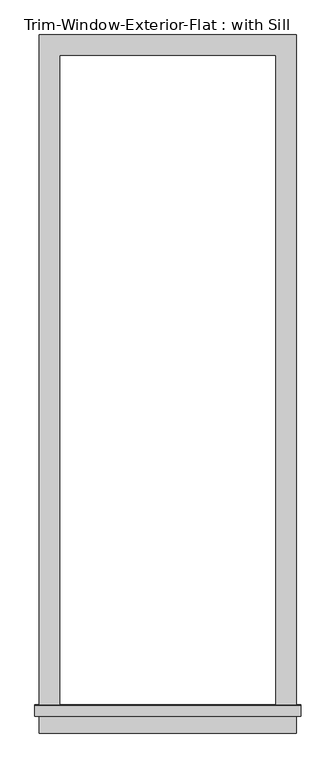
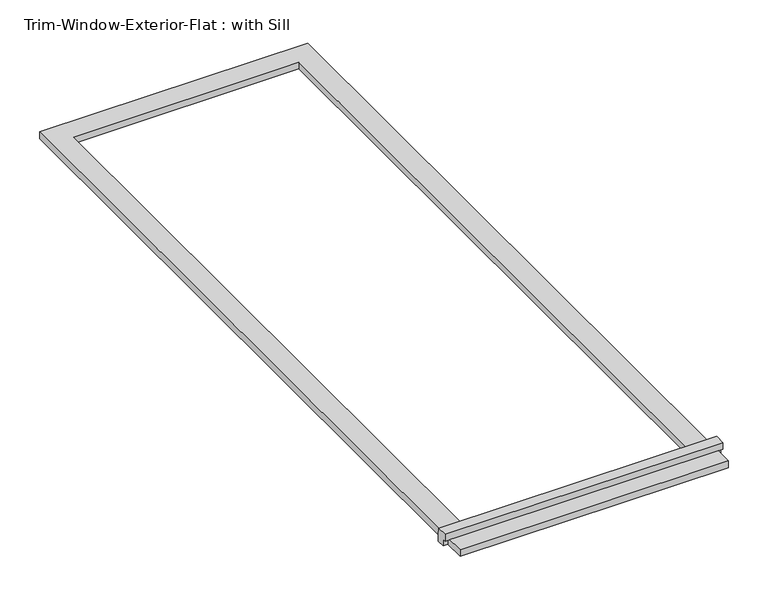
"""IFC4 building model written with IfcOpenShell, lengths in millimetres: proxy geometry, Trim-Window-Exterior-Flat : with Sill."""

from ifc_helpers import new_model, si_unit, frame, origin, origin_with_axes, place, context, project, spatial, polyline, outline, extrude, source, transform, mapped, element, save


def trim_window_exterior_flat_with_sill_19508c7d(model_context):
    return source(origin(), model_context, "Body", "SweptSolid", [
        extrude(outline(polyline([(361.95, -1850.9823709), (361.95, -1908.1323709), (-361.95, -1908.1323709), (-361.95, -1850.9823709), (361.95, -1850.9823709)])), origin_with_axes(), (0.0, 0.0, 1.0), 19.05),
        extrude(outline(polyline([(-1860.55, 38.1), (-1831.2580645, 38.1), (-1828.8, 19.05), (-1828.8, 0.0), (-1850.9823709, 0.0), (-1850.9823709, 19.05), (-1860.55, 19.05), (-1860.55, 38.1)])), frame((-374.65, 0.0, 0.0), z_axis=(1.0, 0.0, 0.0), x_axis=(0.0, 1.0, 0.0)), (0.0, 0.0, 1.0), 749.3),
        extrude(outline(polyline([(-361.95, 57.15), (361.95, 57.15), (361.95, -1828.8), (304.8, -1828.8), (304.8, 0.0), (-304.8, 0.0), (-304.8, -1828.8), (-361.95, -1828.8), (-361.95, 57.15)])), origin_with_axes(), (0.0, 0.0, 1.0), 19.05),
    ])


if __name__ == "__main__":
    model = new_model("IFC4")
    model_context = context("Model", 3, world=origin())
    ifc_project = project(units=[si_unit("LENGTHUNIT", "METRE", prefix="MILLI")], contexts=[model_context])
    site = spatial("IfcSite", under=ifc_project)
    building = spatial("IfcBuilding", under=site)
    placement = place(None, origin())
    trim_window_exterior_flat_with_sill_shape = trim_window_exterior_flat_with_sill_19508c7d(model_context)
    element("IfcBuildingElementProxy", 1, Name="Trim-Window-Exterior-Flat : with Sill", ObjectType="Trim-Window-Exterior-Flat : with Sill", at=placement, inside=building, context=model_context, shape_type="MappedRepresentation", body=[
        mapped(trim_window_exterior_flat_with_sill_shape, transform((0.0, 0.0, 0.0), x_axis=(1.0, 0.0, 0.0), y_axis=(0.0, 1.0, 0.0), z_axis=(0.0, 0.0, 1.0))),
    ])
    save(model, "model.ifc")

# Revit data of these elements
# Type "Trim-Window-Exterior-Flat : with Sill"
#   Trim Width = 0' - 2 1/4"
#   Trim Thickness_Picture Frame = 0' - 1 1/4"
#   Trim Thickness_with Sill = 0' - 0 3/4"
#   Sill Thickness = 0' - 1 1/4"
#   Opening Width [instance default] = 2' - 0"
#   Opening Height [instance default] = 3' - 0"
#   Default Elevation = 4' - 0"
#   Sill = yes
#   Picture Frame = no
#   Trim Material [instance default] = none
# Element 1 (IfcBuildingElementProxy, "Trim-Window-Exterior-Flat : with Sill")
#   Opening Height = 6' - 0"
#   Trim Material = Clad - White
#   Materials on its faces: "Clad - White"
# Materials
#   "Clad - White": class "Wood", colour RGB 242 242 238, transparency 0, Cost = 0
